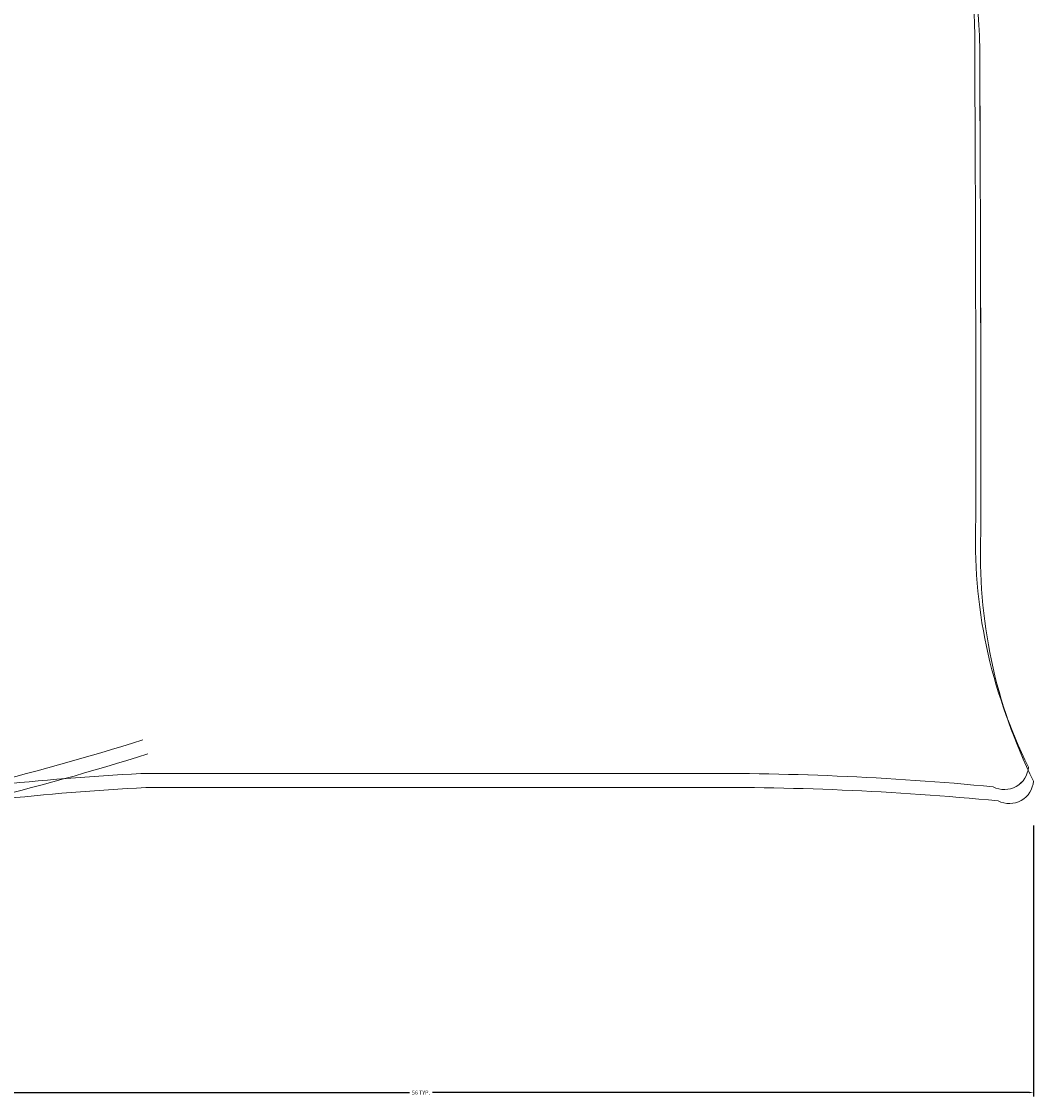
# Model space of a CAD drawing. Units: inches. Extents: x 1885 to 2748, y 783 to 2421.
# Tile 98 of 117: x 2395 to 2441, y 2253 to 2302. Entities that reach past the tile are written whole.
import ezdxf

# ---------------------------------------------------------------- set-up
doc = ezdxf.new("R2010")
doc.units = ezdxf.units.IN
doc.layers.add('A-ANNO-DIMS', color=2, linetype='Continuous', lineweight=18)
doc.layers.add('A-FURN', color=8, linetype='Continuous', lineweight=13)
doc.styles.get("Standard").update_dxf_attribs({"font": 'arial.ttf'})
doc.dimstyles.get("Standard").update_dxf_attribs({"dimtxt": 0.18, "dimasz": 0.18, "dimexe": 0.18, "dimexo": 0.0625, "dimgap": 0.09, "dimtad": 0, "dimtih": 1, "dimtoh": 1, "dimdec": 4, "dimzin": 0, "dimdsep": 46, "dimtxsty": 'Standard', "dimcen": 0.09, "dimadec": 0, "dimazin": 0, "dimtfac": 1, "dimtdec": 4, "dimtofl": 0, "dimtmove": 0, "dimatfit": 3, "dimfxl": 1, "dimtolj": 1, "dimtzin": 0, "dimarcsym": 0})

# ---------------------------------------------------------------- blocks, each defined once
blk = doc.blocks.new('BED-DOUBLE')
for p, q in [((79.888, 15.29), (79.888, 39.904)), ((79.888, 15.29), (79.888, 39.904)), ((79.249, 15.062), (79.249, 39.676)), ((79.249, 15.062), (79.249, 39.676))]:
    blk.add_line(p, q)
for centre, radius, start, end in [((68.67, 76.156), 23.065, 267.4714, 296.4681), ((68.67, 76.156), 23.065, 267.4714, 296.4681), ((69.309, 76.384), 23.065, 267.4714, 296.4681), ((69.309, 76.384), 23.065, 267.4714, 296.4681), ((78.874, 54.409), 1.102, 332.6588, 86.02), ((78.874, 54.408), 1.102, 332.6588, 86.02), ((79.513, 54.637), 1.102, 332.6588, 86.02), ((79.513, 54.637), 1.102, 332.6588, 86.02), ((212.92, 41.379), 133.04, 174.4998, 180.63509), ((212.92, 41.379), 133.04, 174.4998, 180.63509), ((212.28, 41.151), 133.04, 174.4998, 180.63509), ((212.28, 41.15), 133.04, 174.4998, 180.63509), ((36.319, 182.264), 129.499, 266.97912, 273.83645), ((36.958, 182.493), 129.499, 266.97912, 273.83645), ((36.958, 182.493), 129.499, 266.97912, 273.83645), ((67.825, -4508.745), 4561.858, 90.002168, 90.286887), ((67.825, -4508.745), 4561.858, 90.002168, 90.286887), ((68.464, -4508.516), 4561.858, 90.002168, 90.286887), ((68.464, -4508.517), 4561.858, 90.002168, 90.286887), ((-23.069, -16.995), 106.459, 13.38322, 17.70533), ((-23.069, -16.995), 106.459, 13.38322, 17.70533), ((201.48, 21.654), 121.759, 182.99578, 189.40907), ((201.48, 21.654), 121.759, 182.99578, 189.40907), ((-23.708, -17.223), 106.459, 13.38322, 17.70533), ((-23.708, -17.223), 106.459, 13.38322, 17.70533), ((200.841, 21.425), 121.759, 182.99578, 189.40907), ((200.841, 21.425), 121.759, 182.99578, 189.40907)]:
    blk.add_arc(centre, radius, start, end)
blk = doc.blocks.new('*D28')
at = {"layer": 'A-ANNO-DIMS', "color": 0, "lineweight": -2, "transparency": 16777216}
for p, q in [((2385.141, 2265.038), (2385.141, 2252.688)), ((2440.966, 2265.038), (2440.966, 2252.688)), ((2385.321, 2252.868), (2412.525, 2252.868)), ((2440.786, 2252.868), (2413.581, 2252.868))]:
    blk.add_line(p, q, dxfattribs=at)
at = {"layer": 'A-ANNO-DIMS', "color": 0, "transparency": 16777216}
for points in [[(2385.321, 2252.898), (2385.321, 2252.838), (2385.141, 2252.868)], [(2440.786, 2252.898), (2440.786, 2252.838), (2440.966, 2252.868)]]:
    blk.add_solid(points, dxfattribs=at)
at = {"layer": 'Defpoints', "color": 0, "transparency": 16777216}
for p in [(2385.141, 2265.1), (2440.966, 2265.1), (2440.966, 2252.868)]:
    blk.add_point(p, dxfattribs=at)
at = {"layer": 'A-ANNO-DIMS', "color": 0, "transparency": 16777216, "insert": (2413.053, 2252.868), "char_height": 0.18, "attachment_point": 5}
blk.add_mtext('\\A1;56 TYP.', dxfattribs=at)

msp = doc.modelspace()

# ---------------------------------------------------------------- block references
at = {"layer": 'A-FURN', "rotation": 269.9999998331857}
msp.add_blockref('BED-DOUBLE', (2385.229, 2346.652), dxfattribs=at)

# ---------------------------------------------------------------- dimensions: what is measured, and where the dimension line sits
at = {"layer": 'A-ANNO-DIMS'}
dim = msp.add_linear_dim(base=(2440.966, 2252.868), p1=(2385.141, 2265.1), p2=(2440.966, 2265.1), angle=360, text='<> TYP.', dimstyle='Standard', override={"dimdec": 0, "dimlfac": 1, "dimrnd": 0, "dimzin": 0, "dimdsep": 46, "dimlunit": 2}, dxfattribs=at)
dim.commit()
dim.dimension.update_dxf_attribs({"geometry": '*D28', "text_midpoint": (2413.053, 2252.868)})

doc.saveas('drawing.dxf')
